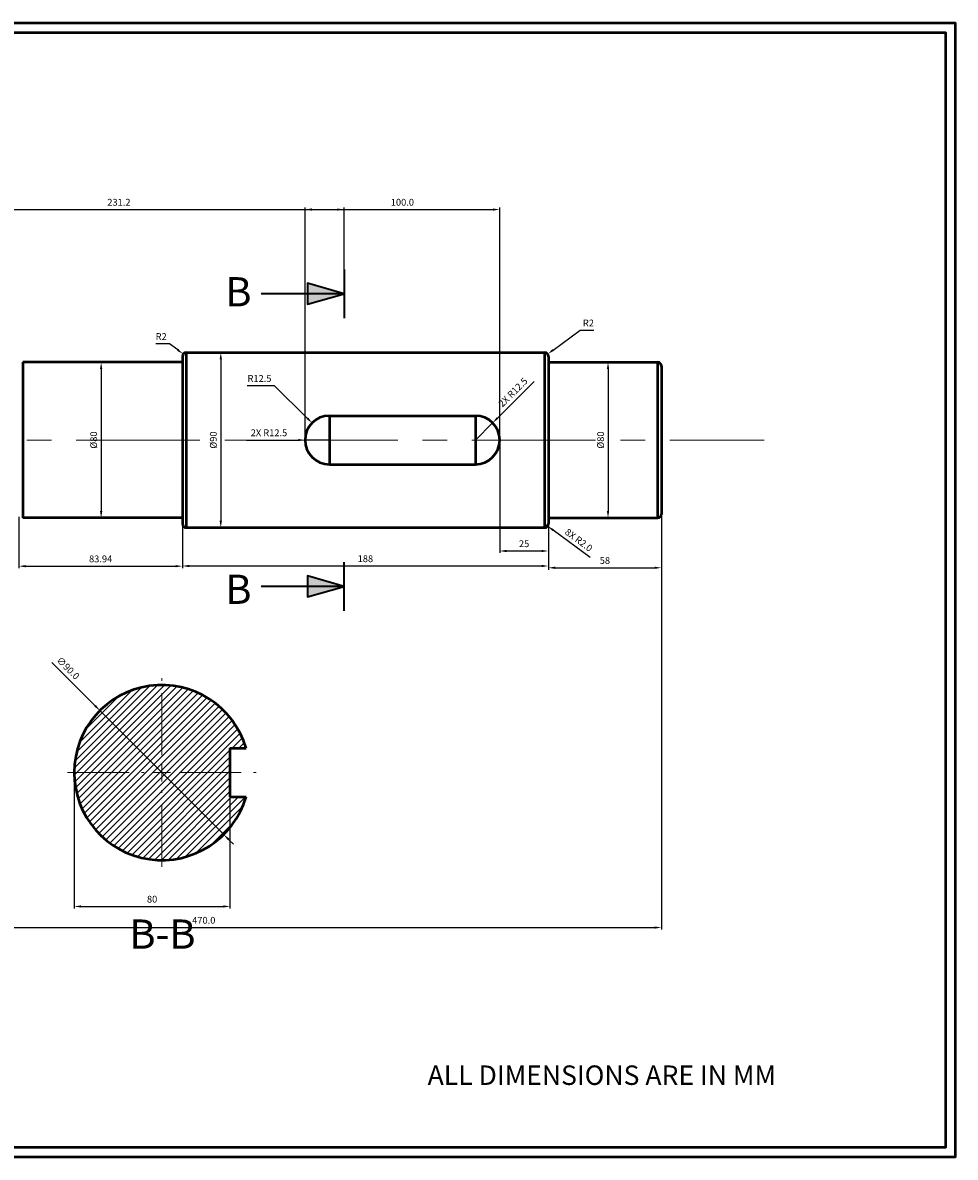
# Model space of a CAD drawing. Units: millimetres. Extents: x 4169 to 4949, y 2556 to 3139.
# Tile 2 of 2: x 4470 to 4949, y 2556 to 3139. Entities that reach past the tile are written whole.
import ezdxf

# ---------------------------------------------------------------- set-up
doc = ezdxf.new("R2010")
doc.units = ezdxf.units.MM
doc.linetypes.add('CENTER', pattern=[50.8, 31.75, -6.35, 6.35, -6.35])
for name, color, linetype, lineweight in [('M-CNTR', 1, 'CENTER', 18), ('M-DIMS', 3, 'Continuous', 25), ('M-HATC', 8, 'Continuous', 18), ('M-OUTL', 7, 'Continuous', 50), ('M-SECT', 7, 'Continuous', 35), ('M-TEXT', 7, 'Continuous', 25), ('M-TTLB', 7, 'Continuous', 50)]:
    doc.layers.add(name, color=color, linetype=linetype, lineweight=lineweight)
doc.styles.get("Standard").update_dxf_attribs({"font": 'arial.ttf'})
doc.dimstyles.new('AM_ISO$0', dxfattribs={"dimtxt": 3.5, "dimasz": 3.5, "dimexe": 1, "dimexo": 1, "dimgap": 1.5, "dimtad": 1, "dimdsep": 46, "dimtxsty": 'Standard', "dimcen": 0, "dimclrd": 256, "dimclre": 256, "dimclrt": 2, "dimadec": 0, "dimazin": 2, "dimtp": 0.1, "dimtm": 0.1, "dimtfac": 0.71, "dimtdec": 3, "dimtmove": 0, "dimatfit": 3, "dimfxl": 1, "dimlwd": -1, "dimlwe": -1, "dimarcsym": 1})
doc.dimstyles.new('AM_ISO$4', dxfattribs={"dimtxt": 3.5, "dimasz": 3.5, "dimexe": 1, "dimexo": 1, "dimgap": 1.5, "dimtad": 1, "dimtoh": 1, "dimdsep": 46, "dimtxsty": 'Standard', "dimcen": 0, "dimclrd": 256, "dimclre": 256, "dimclrt": 2, "dimadec": 0, "dimazin": 2, "dimtp": 0.1, "dimtm": 0.1, "dimtfac": 0.71, "dimtdec": 3, "dimtofl": 0, "dimtmove": 0, "dimatfit": 0, "dimfxl": 1, "dimlwd": -1, "dimlwe": -1, "dimarcsym": 1})

# ---------------------------------------------------------------- blocks, each defined once
blk = doc.blocks.new('*D3')
at = {"layer": 'Defpoints', "color": 0, "transparency": 16777216}
for p in [(4618.26, 2933.8), (4627.14, 2925.01)]:
    blk.add_point(p, dxfattribs=at)
at = {"layer": 'M-DIMS', "color": 0, "linetype": 'ByBlock', "transparency": 16777216}
for p, q in [((4598.97, 2952.9), (4585, 2952.9)), ((4615.77, 2936.26), (4598.97, 2952.9))]:
    blk.add_line(p, q, dxfattribs=at)
at = {"layer": 'M-DIMS', "color": 0, "transparency": 16777216}
blk.add_solid([(4616.18, 2936.68), (4615.36, 2935.85), (4618.26, 2933.8)], dxfattribs=at)
at = {"layer": 'M-DIMS', "color": 0, "transparency": 16777216, "insert": (4591.24, 2956.19), "char_height": 3.5, "attachment_point": 5}
blk.add_mtext('R12.5', dxfattribs=at)
blk = doc.blocks.new('*D5')
at = {"layer": 'Defpoints', "color": 0, "transparency": 16777216}
for p in [(4737.64, 2968.01), (4739.25, 2969.19)]:
    blk.add_point(p, dxfattribs=at)
at = {"layer": 'M-DIMS', "color": 0, "linetype": 'ByBlock', "transparency": 16777216}
for p, q in [((4742.07, 2971.27), (4755.87, 2981.43)), ((4755.87, 2981.43), (4762.98, 2981.43))]:
    blk.add_line(p, q, dxfattribs=at)
at = {"layer": 'M-DIMS', "color": 0, "transparency": 16777216}
blk.add_solid([(4741.73, 2971.74), (4742.42, 2970.8), (4739.25, 2969.19)], dxfattribs=at)
at = {"layer": 'M-DIMS', "color": 0, "transparency": 16777216, "insert": (4760.17, 2984.69), "char_height": 3.5, "attachment_point": 5}
blk.add_mtext('R2', dxfattribs=at)
blk = doc.blocks.new('*D6')
at = {"layer": 'Defpoints', "color": 0, "transparency": 16777216}
for p in [(4552.05, 2969.21), (4553.64, 2968.01)]:
    blk.add_point(p, dxfattribs=at)
at = {"layer": 'M-DIMS', "color": 0, "linetype": 'ByBlock', "transparency": 16777216}
for p, q in [((4545.05, 2974.47), (4537.94, 2974.47)), ((4549.25, 2971.31), (4545.05, 2974.47))]:
    blk.add_line(p, q, dxfattribs=at)
at = {"layer": 'M-DIMS', "color": 0, "transparency": 16777216}
blk.add_solid([(4549.6, 2971.78), (4548.9, 2970.85), (4552.05, 2969.21)], dxfattribs=at)
at = {"layer": 'M-DIMS', "color": 0, "transparency": 16777216, "insert": (4540.74, 2977.73), "char_height": 3.5, "attachment_point": 5}
blk.add_mtext('R2', dxfattribs=at)
blk = doc.blocks.new('*D11')
at = {"layer": 'Defpoints', "color": 0, "transparency": 16777216}
for p in [(4467.7, 2886.53), (4551.64, 2882.01), (4551.64, 2860.2)]:
    blk.add_point(p, dxfattribs=at)
at = {"layer": 'M-DIMS', "color": 0, "linetype": 'ByBlock', "transparency": 16777216}
for p, q in [((4467.7, 2885.53), (4467.7, 2859.2)), ((4551.64, 2881.01), (4551.64, 2859.2)), ((4471.2, 2860.2), (4548.14, 2860.2))]:
    blk.add_line(p, q, dxfattribs=at)
at = {"layer": 'M-DIMS', "color": 0, "transparency": 16777216}
for points in [[(4471.2, 2860.79), (4471.2, 2859.62), (4467.7, 2860.2)], [(4548.14, 2860.79), (4548.14, 2859.62), (4551.64, 2860.2)]]:
    blk.add_solid(points, dxfattribs=at)
at = {"layer": 'M-DIMS', "color": 0, "transparency": 16777216, "insert": (4509.67, 2863.49), "char_height": 3.5, "attachment_point": 5}
blk.add_mtext('83.94', dxfattribs=at)
blk = doc.blocks.new('*D12')
at = {"layer": 'Defpoints', "color": 0, "transparency": 16777216}
for p in [(4551.64, 2882.01), (4739.64, 2882.01), (4739.64, 2860.3)]:
    blk.add_point(p, dxfattribs=at)
at = {"layer": 'M-DIMS', "color": 0, "linetype": 'ByBlock', "transparency": 16777216}
for p, q in [((4551.64, 2881.01), (4551.64, 2859.3)), ((4739.64, 2881.01), (4739.64, 2859.3)), ((4555.14, 2860.3), (4736.14, 2860.3))]:
    blk.add_line(p, q, dxfattribs=at)
at = {"layer": 'M-DIMS', "color": 0, "transparency": 16777216}
for points in [[(4555.14, 2860.89), (4555.14, 2859.72), (4551.64, 2860.3)], [(4736.14, 2860.89), (4736.14, 2859.72), (4739.64, 2860.3)]]:
    blk.add_solid(points, dxfattribs=at)
at = {"layer": 'M-DIMS', "color": 0, "transparency": 16777216, "insert": (4645.64, 2863.59), "char_height": 3.5, "attachment_point": 5}
blk.add_mtext('188', dxfattribs=at)
blk = doc.blocks.new('*D13')
at = {"layer": 'Defpoints', "color": 0, "transparency": 16777216}
for p in [(4797.64, 2887.01), (4739.64, 2885.01), (4797.64, 2859.39)]:
    blk.add_point(p, dxfattribs=at)
at = {"layer": 'M-DIMS', "color": 0, "linetype": 'ByBlock', "transparency": 16777216}
for p, q in [((4797.64, 2886.01), (4797.64, 2858.39)), ((4739.64, 2884.01), (4739.64, 2858.39)), ((4743.14, 2859.39), (4794.14, 2859.39))]:
    blk.add_line(p, q, dxfattribs=at)
at = {"layer": 'M-DIMS', "color": 0, "transparency": 16777216}
for points in [[(4743.14, 2859.97), (4743.14, 2858.8), (4739.64, 2859.39)], [(4794.14, 2859.97), (4794.14, 2858.8), (4797.64, 2859.39)]]:
    blk.add_solid(points, dxfattribs=at)
at = {"layer": 'M-DIMS', "color": 0, "transparency": 16777216, "insert": (4768.64, 2862.67), "char_height": 3.5, "attachment_point": 5}
blk.add_mtext('58', dxfattribs=at)
blk = doc.blocks.new('*D15')
at = {"layer": 'Defpoints', "color": 0, "transparency": 16777216}
for p in [(4491.54, 2965.01), (4491.54, 2885.01), (4509.94, 2885.01)]:
    blk.add_point(p, dxfattribs=at)
at = {"layer": 'M-DIMS', "color": 0, "linetype": 'ByBlock', "transparency": 16777216}
for p, q in [((4492.54, 2965.01), (4510.94, 2965.01)), ((4509.94, 2961.51), (4509.94, 2888.51)), ((4492.54, 2885.01), (4510.94, 2885.01))]:
    blk.add_line(p, q, dxfattribs=at)
at = {"layer": 'M-DIMS', "color": 0, "transparency": 16777216}
for points in [[(4509.35, 2961.51), (4510.52, 2961.51), (4509.94, 2965.01)], [(4509.35, 2888.51), (4510.52, 2888.51), (4509.94, 2885.01)]]:
    blk.add_solid(points, dxfattribs=at)
at = {"layer": 'M-DIMS', "color": 0, "transparency": 16777216, "insert": (4506.55, 2925.01), "char_height": 3.5, "attachment_point": 5, "rotation": 90}
blk.add_mtext('%%C80', dxfattribs=at)
blk = doc.blocks.new('*D16')
at = {"layer": 'Defpoints', "color": 0, "transparency": 16777216}
for p in [(4578.11, 2970.01), (4571.38, 2880.01), (4578.11, 2880.01)]:
    blk.add_point(p, dxfattribs=at)
at = {"layer": 'M-DIMS', "color": 0, "linetype": 'ByBlock', "transparency": 16777216}
for p, q in [((4577.11, 2970.01), (4570.38, 2970.01)), ((4571.38, 2966.51), (4571.38, 2883.51)), ((4577.11, 2880.01), (4570.38, 2880.01))]:
    blk.add_line(p, q, dxfattribs=at)
at = {"layer": 'M-DIMS', "color": 0, "transparency": 16777216}
for points in [[(4570.79, 2966.51), (4571.96, 2966.51), (4571.38, 2970.01)], [(4570.79, 2883.51), (4571.96, 2883.51), (4571.38, 2880.01)]]:
    blk.add_solid(points, dxfattribs=at)
at = {"layer": 'M-DIMS', "color": 0, "transparency": 16777216, "insert": (4567.99, 2925.01), "char_height": 3.5, "attachment_point": 5, "rotation": 90}
blk.add_mtext('%%C90', dxfattribs=at)
blk = doc.blocks.new('*D17')
at = {"layer": 'Defpoints', "color": 0, "transparency": 16777216}
for p in [(4766.65, 2965.01), (4766.65, 2885.01), (4770.24, 2885.01)]:
    blk.add_point(p, dxfattribs=at)
at = {"layer": 'M-DIMS', "color": 0, "linetype": 'ByBlock', "transparency": 16777216}
for p, q in [((4767.65, 2965.01), (4771.24, 2965.01)), ((4770.24, 2961.51), (4770.24, 2888.51)), ((4767.65, 2885.01), (4771.24, 2885.01))]:
    blk.add_line(p, q, dxfattribs=at)
at = {"layer": 'M-DIMS', "color": 0, "transparency": 16777216}
for points in [[(4769.66, 2961.51), (4770.82, 2961.51), (4770.24, 2965.01)], [(4769.66, 2888.51), (4770.82, 2888.51), (4770.24, 2885.01)]]:
    blk.add_solid(points, dxfattribs=at)
at = {"layer": 'M-DIMS', "color": 0, "transparency": 16777216, "insert": (4766.86, 2925.01), "char_height": 3.5, "attachment_point": 5, "rotation": 90}
blk.add_mtext('%%C80', dxfattribs=at)
blk = doc.blocks.new('*D18')
at = {"layer": 'Defpoints', "color": 0, "transparency": 16777216}
for p in [(4714.64, 2925.01), (4739.64, 2925.01), (4739.64, 2868.01)]:
    blk.add_point(p, dxfattribs=at)
at = {"layer": 'M-DIMS', "color": 0, "linetype": 'ByBlock', "transparency": 16777216}
for p, q in [((4714.64, 2924.01), (4714.64, 2867.01)), ((4739.64, 2924.01), (4739.64, 2867.01)), ((4718.14, 2868.01), (4736.14, 2868.01))]:
    blk.add_line(p, q, dxfattribs=at)
at = {"layer": 'M-DIMS', "color": 0, "transparency": 16777216}
for points in [[(4718.14, 2868.59), (4718.14, 2867.42), (4714.64, 2868.01)], [(4736.14, 2868.59), (4736.14, 2867.42), (4739.64, 2868.01)]]:
    blk.add_solid(points, dxfattribs=at)
at = {"layer": 'M-DIMS', "color": 0, "transparency": 16777216, "insert": (4727.14, 2871.29), "char_height": 3.5, "attachment_point": 5}
blk.add_mtext('25', dxfattribs=at)
blk = doc.blocks.new('*U22')
at = {"layer": 'M-CNTR', "color": 0, "transparency": 16777216}
for p, q in [((0, 9), (0, 48.5)), ((-48.5, 0), (-9, 0)), ((9, 0), (48.5, 0)), ((0, -48.5), (0, -9))]:
    blk.add_line(p, q, dxfattribs=at)
at = {"layer": 'M-CNTR', "color": 0, "linetype": 'Continuous', "transparency": 16777216}
for p, q in [((-4.5, 0), (4.5, 0)), ((0, -4.5), (0, 4.5))]:
    blk.add_line(p, q, dxfattribs=at)
blk = doc.blocks.new('*D23')
at = {"layer": 'Defpoints', "color": 0, "transparency": 16777216}
for p in [(4496.1, 2754.16), (4576.1, 2754.16), (4576.1, 2685.37)]:
    blk.add_point(p, dxfattribs=at)
at = {"layer": 'M-DIMS', "color": 0, "linetype": 'ByBlock', "transparency": 16777216}
for p, q in [((4496.1, 2753.16), (4496.1, 2684.37)), ((4576.1, 2753.16), (4576.1, 2684.37)), ((4499.6, 2685.37), (4572.6, 2685.37))]:
    blk.add_line(p, q, dxfattribs=at)
at = {"layer": 'M-DIMS', "color": 0, "transparency": 16777216}
for points in [[(4499.6, 2685.95), (4499.6, 2684.79), (4496.1, 2685.37)], [(4572.6, 2685.95), (4572.6, 2684.79), (4576.1, 2685.37)]]:
    blk.add_solid(points, dxfattribs=at)
at = {"layer": 'M-DIMS', "color": 0, "transparency": 16777216, "insert": (4536.1, 2688.66), "char_height": 3.5, "attachment_point": 5}
blk.add_mtext('80', dxfattribs=at)
blk = doc.blocks.new('*D24')
at = {"layer": 'Defpoints', "color": 0, "transparency": 16777216}
for p in [(4327.64, 2892.01), (4797.64, 2887.01), (4797.64, 2674.52)]:
    blk.add_point(p, dxfattribs=at)
at = {"layer": 'M-DIMS', "linetype": 'ByBlock', "transparency": 16777216}
for p, q in [((4327.64, 2891.01), (4327.64, 2673.52)), ((4797.64, 2886.01), (4797.64, 2673.52)), ((4331.14, 2674.52), (4794.14, 2674.52))]:
    blk.add_line(p, q, dxfattribs=at)
at = {"layer": 'M-DIMS', "transparency": 16777216}
for points in [[(4331.14, 2675.11), (4331.14, 2673.94), (4327.64, 2674.52)], [(4794.14, 2675.11), (4794.14, 2673.94), (4797.64, 2674.52)]]:
    blk.add_solid(points, dxfattribs=at)
at = {"layer": 'M-DIMS', "color": 2, "transparency": 16777216, "insert": (4562.64, 2677.81), "char_height": 3.5, "attachment_point": 5}
blk.add_mtext('470.0', dxfattribs=at)
blk = doc.blocks.new('*D25')
at = {"layer": 'Defpoints', "color": 0, "transparency": 16777216}
for p in [(4714.64, 3043.44), (4614.64, 2925.01), (4714.64, 2925.01)]:
    blk.add_point(p, dxfattribs=at)
at = {"layer": 'M-DIMS', "linetype": 'ByBlock', "transparency": 16777216}
for p, q in [((4614.64, 2926.01), (4614.64, 3044.44)), ((4618.14, 3043.44), (4711.14, 3043.44)), ((4714.64, 2926.01), (4714.64, 3044.44))]:
    blk.add_line(p, q, dxfattribs=at)
at = {"layer": 'M-DIMS', "transparency": 16777216}
for points in [[(4618.14, 3044.02), (4618.14, 3042.86), (4614.64, 3043.44)], [(4711.14, 3044.02), (4711.14, 3042.86), (4714.64, 3043.44)]]:
    blk.add_solid(points, dxfattribs=at)
at = {"layer": 'M-DIMS', "color": 2, "transparency": 16777216, "insert": (4664.64, 3046.73), "char_height": 3.5, "attachment_point": 5}
blk.add_mtext('100.0', dxfattribs=at)
blk = doc.blocks.new('*D27')
at = {"layer": 'Defpoints', "color": 0, "transparency": 16777216}
for p in [(4634.66, 3043.44), (4403.47, 3002.69), (4634.66, 3000.19)]:
    blk.add_point(p, dxfattribs=at)
at = {"layer": 'M-DIMS', "linetype": 'ByBlock', "transparency": 16777216}
for p, q in [((4403.47, 3003.69), (4403.47, 3044.44)), ((4406.97, 3043.44), (4631.16, 3043.44)), ((4634.66, 3001.19), (4634.66, 3044.44))]:
    blk.add_line(p, q, dxfattribs=at)
at = {"layer": 'M-DIMS', "transparency": 16777216}
for points in [[(4406.97, 3044.02), (4406.97, 3042.86), (4403.47, 3043.44)], [(4631.16, 3044.02), (4631.16, 3042.86), (4634.66, 3043.44)]]:
    blk.add_solid(points, dxfattribs=at)
at = {"layer": 'M-DIMS', "color": 2, "transparency": 16777216, "insert": (4519.06, 3046.73), "char_height": 3.5, "attachment_point": 5}
blk.add_mtext('231.2', dxfattribs=at)
blk = doc.blocks.new('*D29')
at = {"layer": 'Defpoints', "color": 0, "transparency": 16777216}
for p in [(4710.99, 2933.84), (4702.14, 2925.01)]:
    blk.add_point(p, dxfattribs=at)
at = {"layer": 'M-DIMS', "linetype": 'ByBlock', "transparency": 16777216}
for p, q in [((4732.24, 2955.08), (4713.46, 2936.32)), ((4702.14, 2925.01), (4710.99, 2933.84))]:
    blk.add_line(p, q, dxfattribs=at)
at = {"layer": 'M-DIMS', "transparency": 16777216}
blk.add_solid([(4713.05, 2936.73), (4713.87, 2935.9), (4710.99, 2933.84)], dxfattribs=at)
at = {"layer": 'M-DIMS', "color": 2, "transparency": 16777216, "insert": (4721.76, 2949.26), "char_height": 3.5, "attachment_point": 5, "rotation": 44.98473}
blk.add_mtext('2X R12.5', dxfattribs=at)
blk = doc.blocks.new('*D30')
at = {"layer": 'Defpoints', "color": 0, "transparency": 16777216}
for p in [(4737.64, 2882.01), (4739.25, 2880.81)]:
    blk.add_point(p, dxfattribs=at)
at = {"layer": 'M-DIMS', "linetype": 'ByBlock', "transparency": 16777216}
for p, q in [((4737.64, 2882.01), (4739.25, 2880.81)), ((4761.12, 2864.58), (4742.06, 2878.73))]:
    blk.add_line(p, q, dxfattribs=at)
at = {"layer": 'M-DIMS', "transparency": 16777216}
blk.add_solid([(4742.41, 2879.2), (4741.71, 2878.26), (4739.25, 2880.81)], dxfattribs=at)
at = {"layer": 'M-DIMS', "color": 2, "transparency": 16777216, "insert": (4754.95, 2873.25), "char_height": 3.5, "attachment_point": 5, "rotation": 323.41527}
blk.add_mtext('8X R2.0', dxfattribs=at)
blk = doc.blocks.new('*D31')
at = {"layer": 'Defpoints', "color": 0, "transparency": 16777216}
for p in [(4509.3, 2786), (4572.9, 2722.32)]:
    blk.add_point(p, dxfattribs=at)
at = {"layer": 'M-DIMS', "linetype": 'ByBlock', "transparency": 16777216}
for p, q in [((4484.61, 2810.72), (4506.83, 2788.47)), ((4572.9, 2722.32), (4509.3, 2786)), ((4575.38, 2719.84), (4577.85, 2717.36))]:
    blk.add_line(p, q, dxfattribs=at)
at = {"layer": 'M-DIMS', "transparency": 16777216}
for points in [[(4507.24, 2788.89), (4506.42, 2788.06), (4509.3, 2786)], [(4575.79, 2720.25), (4574.96, 2719.43), (4572.9, 2722.32)]]:
    blk.add_solid(points, dxfattribs=at)
at = {"layer": 'M-DIMS', "color": 2, "transparency": 16777216, "insert": (4492.62, 2807.49), "char_height": 3.5, "attachment_point": 5, "rotation": 314.96412}
blk.add_mtext('∅90.0', dxfattribs=at)
blk = doc.blocks.new('*D35')
at = {"layer": 'Defpoints', "color": 0, "transparency": 16777216}
for p in [(4614.64, 2925.01), (4627.14, 2925.01)]:
    blk.add_point(p, dxfattribs=at)
at = {"layer": 'M-DIMS', "linetype": 'ByBlock', "transparency": 16777216}
for p, q in [((4584.6, 2925.01), (4611.14, 2925.01)), ((4627.14, 2925.01), (4614.64, 2925.01))]:
    blk.add_line(p, q, dxfattribs=at)
at = {"layer": 'M-DIMS', "transparency": 16777216}
blk.add_solid([(4611.14, 2925.59), (4611.14, 2924.42), (4614.64, 2925.01)], dxfattribs=at)
at = {"layer": 'M-DIMS', "color": 2, "transparency": 16777216, "insert": (4596.12, 2928.29), "char_height": 3.5, "attachment_point": 5, "rotation": 359.99801}
blk.add_mtext('2X R12.5', dxfattribs=at)

msp = doc.modelspace()

# ---------------------------------------------------------------- hatches: boundary and pattern name
at = {"layer": 'M-HATC'}
h = msp.add_hatch(dxfattribs=at)
h.set_pattern_fill('_U', color=256, scale=2.5, angle=45, style=0, pattern_type=0)
h.set_pattern_definition([(45, (0, 6.7532), (-1.767767, 1.767767), [])])
edge = h.paths.add_edge_path()
edge.add_line((4584.332, 2741.657), (4576.103, 2741.657))
edge.add_line((4576.103, 2741.657), (4576.103, 2766.657))
edge.add_line((4576.103, 2766.657), (4584.332, 2766.657))
edge.add_arc((4541.103, 2754.157), 45, 16.12762, 343.87238)
at = {"layer": 'M-SECT'}
h = msp.add_hatch(color=256, dxfattribs=at)
h.set_gradient(color1=(0, 0, 255), color2=(255, 255, 0), tint=1, name='CYLINDER')
h.paths.add_polyline_path([(4634.658, 3000.189), (4615.935, 3000.189), (4615.935, 2994.843)])
h.paths.add_polyline_path([(4615.935, 3005.535), (4615.935, 3000.189), (4634.658, 3000.189)])
h.paths.add_polyline_path([(4615.935, 2855.17), (4615.935, 2849.824), (4634.658, 2849.824)])
h.paths.add_polyline_path([(4634.658, 2849.824), (4615.935, 2849.824), (4615.935, 2844.478)])

# ---------------------------------------------------------------- linework, layer by layer
at = {"layer": 'M-CNTR', "ltscale": 2}
msp.add_line((4293.966, 2925.007), (4850.492, 2925.007), dxfattribs=at)
at = {"layer": 'M-OUTL'}
for p, q in [((4551.644, 2968.007), (4551.644, 2882.007)), ((4553.644, 2970.007), (4553.644, 2880.007)), ((4553.644, 2970.007), (4737.644, 2970.007)), ((4737.644, 2970.007), (4737.644, 2880.007)), ((4739.644, 2968.007), (4739.644, 2882.007)), ((4551.644, 2965.007), (4469.644, 2965.007)), ((4469.644, 2965.007), (4469.644, 2885.007)), ((4469.644, 2965.007), (4469.644, 2963.007)), ((4739.644, 2965.007), (4795.644, 2965.007)), ((4795.644, 2965.007), (4795.644, 2885.007)), ((4797.644, 2963.007), (4797.644, 2887.007)), ((4627.144, 2937.507), (4627.144, 2912.507)), ((4627.144, 2937.507), (4702.144, 2937.507)), ((4702.144, 2937.507), (4702.144, 2912.507)), ((4627.144, 2912.507), (4702.144, 2912.507)), ((4551.644, 2885.007), (4469.644, 2885.007)), ((4553.644, 2880.007), (4737.644, 2880.007)), ((4739.644, 2885.007), (4795.644, 2885.007)), ((4576.103, 2766.657), (4576.103, 2741.657)), ((4576.103, 2766.657), (4584.332, 2766.657)), ((4576.103, 2741.657), (4584.332, 2741.657))]:
    msp.add_line(p, q, dxfattribs=at)
for centre, radius, start, end in [((4553.644, 2968.007), 2, 90, 180), ((4737.644, 2968.007), 2, 0, 90), ((4795.644, 2963.007), 2, 0, 90), ((4627.144, 2925.007), 12.5, 90, 270), ((4702.144, 2925.007), 12.5, 270, 90), ((4795.644, 2887.007), 2, 270, 0), ((4553.644, 2882.007), 2, 180, 270), ((4737.644, 2882.007), 2, 270, 0), ((4541.103, 2754.157), 45, 16.12762, 343.87238)]:
    msp.add_arc(centre, radius, start, end, dxfattribs=at)
at = {"layer": 'M-SECT'}
for p, q in [((4634.658, 3012.689), (4634.658, 2987.689)), ((4634.658, 3000.189), (4592.073, 3000.189)), ((4634.658, 3000.189), (4603.284, 3000.189)), ((4634.658, 2837.324), (4634.658, 2862.324)), ((4634.658, 2849.824), (4592.073, 2849.824))]:
    msp.add_line(p, q, dxfattribs=at)
for points in [[(4634.658, 3000.189), (4615.935, 3005.535), (4615.935, 2994.843)], [(4634.658, 2849.824), (4615.935, 2855.17), (4615.935, 2844.478)]]:
    msp.add_lwpolyline(points, close=True, dxfattribs=at)
at = {"layer": 'M-TTLB'}
for points in [[(4169.043, 3139.451), (4948.587, 3139.451), (4948.587, 2556.482), (4169.043, 2556.482)], [(4174.043, 3134.451), (4943.587, 3134.451), (4943.587, 2561.482), (4174.043, 2561.482)]]:
    msp.add_lwpolyline(points, close=True, dxfattribs=at)

# ---------------------------------------------------------------- block references
at = {"layer": 'M-CNTR'}
msp.add_blockref('*U22', (4541.103, 2754.157), dxfattribs=at)

# ---------------------------------------------------------------- texts
at = {"layer": 'M-TEXT'}
for s, height, p in [('B', 15, (4573.715, 2993.704)), ('B', 15, (4573.715, 2840.834)), ('B-B', 15, (4524.445, 2663.674)), ('ALL DIMENSIONS ARE IN MM ', 10, (4677.599, 2593.67))]:
    msp.add_text(s, height=height, dxfattribs=at).set_placement(p)

# ---------------------------------------------------------------- dimensions: what is measured, and where the dimension line sits
at = {"layer": 'M-DIMS'}
for base, p1, p2, picture, middle in [((4634.658, 3043.439), (4403.47, 3002.689), (4634.658, 3000.189), '*D27', (4519.064, 3046.727)), ((4714.644, 3043.439), (4614.644, 2925.007), (4714.644, 2925.007), '*D25', (4664.644, 3046.726)), ((4797.644, 2674.523), (4327.644, 2892.007), (4797.644, 2887.007), '*D24', (4562.644, 2677.81))]:
    dim = msp.add_linear_dim(base=base, p1=p1, p2=p2, dimstyle='AM_ISO$0', override={"dimdec": 1, "dimlfac": 1, "dimrnd": 0, "dimzin": 0, "dimdsep": 46, "dimlunit": 2}, dxfattribs=at)
    dim.commit()
    dim.dimension.update_dxf_attribs({"geometry": picture, "text_midpoint": middle})
for center, mpoint, override, picture, middle in [((4737.644, 2968.007), (4739.254, 2969.193), {"dimpost": '', "dimclrd": 0, "dimclre": 0, "dimclrt": 0}, '*D5', (4760.174, 2981.434)), ((4553.644, 2968.007), (4552.046, 2969.209), {"dimclrd": 0, "dimclre": 0, "dimclrt": 0}, '*D6', (4540.744, 2974.473)), ((4627.144, 2925.007), (4618.261, 2933.801), {"dimpost": '', "dimclrd": 0, "dimclre": 0, "dimclrt": 0}, '*D3', (4591.235, 2952.899))]:
    dim = msp.add_radius_dim(center=center, mpoint=mpoint, dimstyle='AM_ISO$4', override=override, dxfattribs=at)
    dim.commit()
    dim.dimension.update_dxf_attribs({"geometry": picture, "text_midpoint": middle, "dimtype": 164})
for base, p1, p2, picture, middle in [((4571.376, 2880.007), (4578.108, 2970.007), (4578.108, 2880.007), '*D16', (4567.991, 2925.007)), ((4509.935, 2885.007), (4491.543, 2965.007), (4491.543, 2885.007), '*D15', (4506.55, 2925.007))]:
    dim = msp.add_linear_dim(base=base, p1=p1, p2=p2, angle=90, text='%%C<>', dimstyle='AM_ISO$0', override={"dimpost": '', "dimclrd": 0, "dimclre": 0, "dimclrt": 0}, dxfattribs=at)
    dim.commit()
    dim.dimension.update_dxf_attribs({"geometry": picture, "text_midpoint": middle})
dim = msp.add_linear_dim(base=(4770.24, 2885.007), p1=(4766.654, 2965.007), p2=(4766.654, 2885.007), angle=90, text='%%C<>', dimstyle='AM_ISO$0', override={"dimclrd": 0, "dimclre": 0, "dimclrt": 0}, dxfattribs=at)
dim.commit()
dim.dimension.update_dxf_attribs({"geometry": '*D17', "text_midpoint": (4770.24, 2925.007), "dimtype": 160})
for center, mpoint, text, picture, middle in [((4702.144, 2925.007), (4710.985, 2933.843), '2X <>', '*D29', (4721.763, 2949.263)), ((4627.144, 2925.007), (4614.644, 2925.007), '2X <>', '*D35', (4596.12, 2928.295)), ((4737.644, 2882.007), (4739.25, 2880.815), '8X <>', '*D30', (4754.954, 2873.252))]:
    dim = msp.add_radius_dim(center=center, mpoint=mpoint, text=text, dimstyle='AM_ISO$0', override={"dimdec": 1, "dimlfac": 1, "dimrnd": 0, "dimzin": 0, "dimdsep": 46, "dimlunit": 2}, dxfattribs=at)
    dim.commit()
    dim.dimension.update_dxf_attribs({"geometry": picture, "text_midpoint": middle})
for base, p1, p2, override, picture, middle in [((4739.644, 2868.007), (4714.644, 2925.007), (4739.644, 2925.007), {"dimpost": '', "dimclrd": 0, "dimclre": 0, "dimclrt": 0}, '*D18', (4727.144, 2871.294)), ((4551.644, 2860.204), (4467.701, 2886.531), (4551.644, 2882.007), {"dimpost": '', "dimclrd": 0, "dimclre": 0, "dimclrt": 0}, '*D11', (4509.673, 2863.492)), ((4797.644, 2859.388), (4739.644, 2885.007), (4797.644, 2887.007), {"dimclrd": 0, "dimclre": 0, "dimclrt": 0}, '*D13', (4768.644, 2862.675)), ((4739.644, 2860.305), (4551.644, 2882.007), (4739.644, 2882.007), {"dimpost": '', "dimclrd": 0, "dimclre": 0, "dimclrt": 0}, '*D12', (4645.644, 2863.592)), ((4576.103, 2685.37), (4496.103, 2754.157), (4576.103, 2754.157), {"dimpost": '', "dimclrd": 0, "dimclre": 0, "dimclrt": 0}, '*D23', (4536.103, 2688.657))]:
    dim = msp.add_linear_dim(base=base, p1=p1, p2=p2, angle=0, dimstyle='AM_ISO$0', override=override, dxfattribs=at)
    dim.commit()
    dim.dimension.update_dxf_attribs({"geometry": picture, "text_midpoint": middle})
dim = msp.add_diameter_dim_2p(p1=(4572.903, 2722.318), p2=(4509.303, 2785.997), dimstyle='AM_ISO$0', override={"dimdec": 1, "dimlfac": 1, "dimrnd": 0, "dimzin": 0, "dimdsep": 46, "dimlunit": 2}, dxfattribs=at)
dim.commit()
dim.dimension.update_dxf_attribs({"geometry": '*D31', "text_midpoint": (4490.223, 2805.101), "dimtype": 163})

doc.saveas('drawing.dxf')
